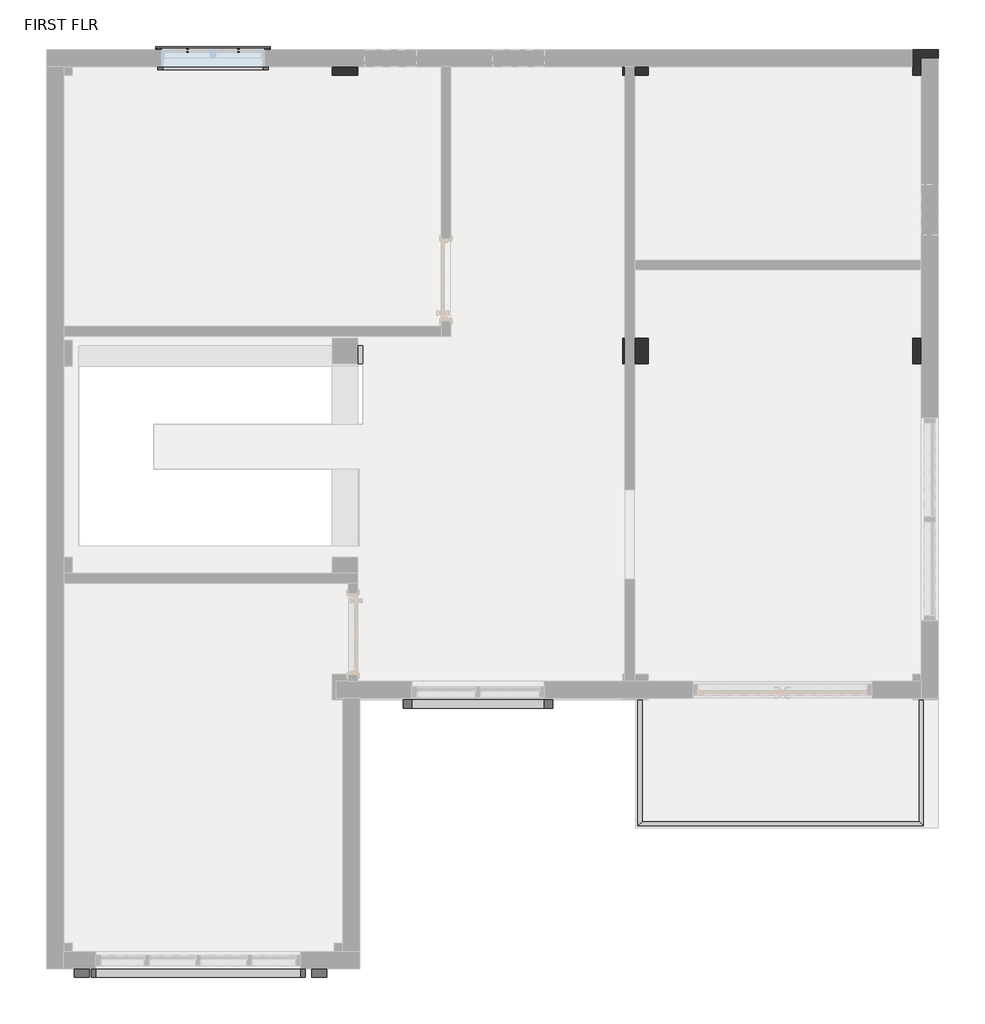
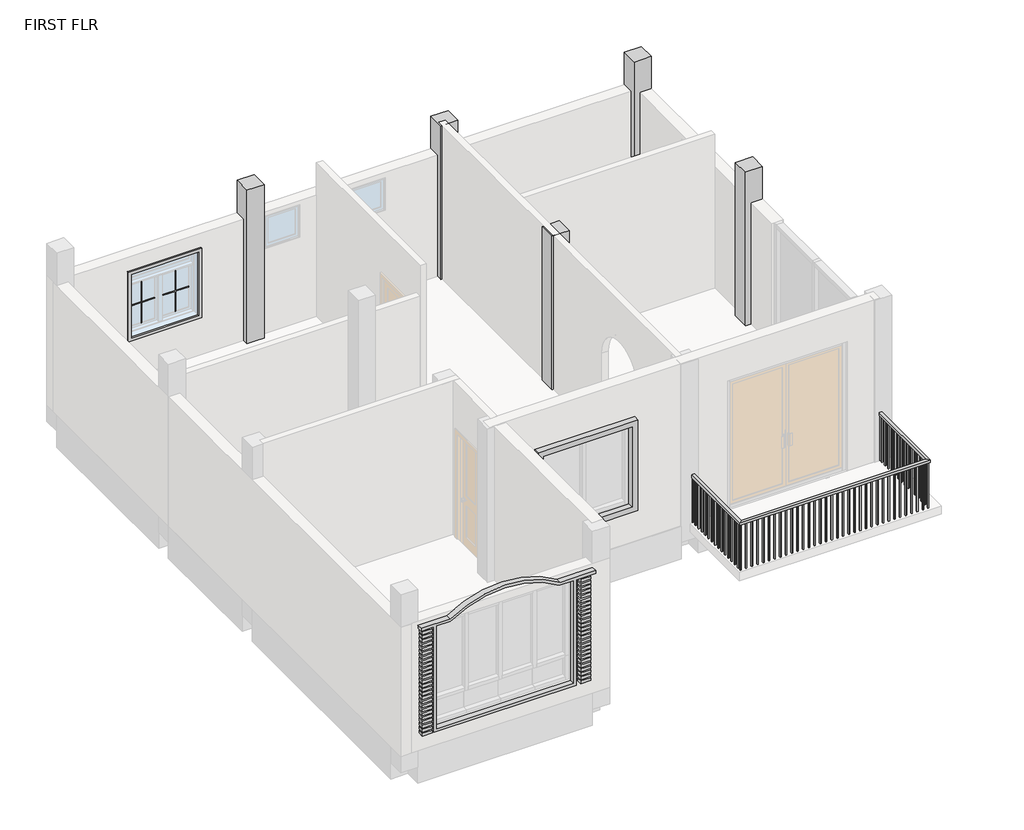
# One storey, part 3 of 3: 7 proxies, 6 beams, 5 columns, 1 railing.
"""IFC4 building model written with IfcOpenShell, lengths in millimetres."""

from ifc_helpers import new_model, si_unit, frame, origin, place, context, project, spatial, polyline, outline, extrude, faceted_brep, transform, mapped, element, save
from components import generic_models_5_generic_models_5_33064adf, generic_models_6_generic_models_6_eab10de4, generic_models_8_generic_models_8_74760410, muntin_pattern_2x2_muntin_pattern_2x2_2357e71d, muntin_pattern_2x2_muntin_pattern_2x2_302d8f29, trim_window_exterior_flat_with_sill_7cfdd449, trim_window_interior_flat_picture_frame_f1e0b15b

model = new_model("IFC4")

# Units and contexts
model_context = context("Model", 3, world=origin())
ifc_project = project(units=[si_unit("LENGTHUNIT", "METRE", prefix="MILLI")], contexts=[model_context])

# Site, building, storey
site = spatial("IfcSite", under=ifc_project)
building = spatial("IfcBuilding", under=site)
storey = spatial("IfcBuildingStorey", under=building, Name="FIRST FLR", Elevation=3352.8)

# Beams
placement = place(None, origin())
element("IfcBeam", 1, ObjectType="Concrete-Rectangular Beam : 12 x 24", at=placement, inside=storey, context=model_context, shape_type="Brep", body=[
    faceted_brep([(-4797.1270642, -2868.8747117, 3352.8), (-4797.1270642, -2564.0747117, 3352.8), (-7946.7270642, -2564.0747117, 3352.8), (-7946.7270642, -2868.8747117, 3352.8), (-4797.1270642, -2868.8747117, 2743.2), (-4797.1270642, -2868.8747117, 3048.0), (-7946.7270642, -2868.8747117, 3048.0), (-7946.7270642, -2868.8747117, 2743.2), (-4797.1270642, -2564.0747117, 2743.2), (-7946.7270642, -2564.0747117, 2743.2), (-4797.1270642, -2564.0747117, 3048.0), (-7946.7270642, -2564.0747117, 3048.0)], [[[0, 1, 2, 3]], [[4, 5, 0, 3, 6, 7]], [[8, 4, 7, 9]], [[1, 10, 8, 9, 11, 2]], [[2, 11, 9, 7, 6, 3]], [[1, 0, 5, 4, 8, 10]]]),
])
element("IfcBeam", 2, ObjectType="Concrete-Rectangular Beam : 12 x 24", at=placement, inside=storey, context=model_context, shape_type="Brep", body=[
    faceted_brep([(-1351.9658472, -2868.8747117, 3352.8), (-1351.9658472, -2564.0747117, 3352.8), (-4492.3270642, -2564.0747117, 3352.8), (-4492.3270642, -2868.8747117, 3352.8), (-1351.9658472, -2868.8747117, 2743.2), (-1351.9658472, -2868.8747117, 3048.0), (-4492.3270642, -2868.8747117, 3048.0), (-4492.3270642, -2868.8747117, 2743.2), (-1351.9658472, -2564.0747117, 2743.2), (-4492.3270642, -2564.0747117, 2743.2), (-1351.9658472, -2564.0747117, 3048.0), (-4492.3270642, -2564.0747117, 3048.0)], [[[0, 1, 2, 3]], [[4, 5, 0, 3, 6, 7]], [[8, 4, 7, 9]], [[1, 10, 8, 9, 11, 2]], [[2, 11, 9, 7, 6, 3]], [[1, 0, 5, 4, 8, 10]]]),
])
element("IfcBeam", 3, ObjectType="Concrete-Rectangular Beam : 12 x 24", at=placement, inside=storey, context=model_context, shape_type="Brep", body=[
    faceted_brep([(-1351.9658472, -5993.0747117, 3352.8), (-1047.1658472, -5993.0747117, 3352.8), (-1047.1658472, -2868.8747117, 3352.8), (-1351.9658472, -2868.8747117, 3352.8), (-1351.9658472, -5993.0747117, 2743.2), (-1351.9658472, -5993.0747117, 3048.0), (-1351.9658472, -2868.8747117, 3048.0), (-1351.9658472, -2868.8747117, 2743.2), (-1047.1658472, -5993.0747117, 2743.2), (-1047.1658472, -2868.8747117, 2743.2), (-1047.1658472, -5993.0747117, 3048.0), (-1047.1658472, -2868.8747117, 3048.0)], [[[0, 1, 2, 3]], [[4, 5, 0, 3, 6, 7]], [[8, 4, 7, 9]], [[1, 10, 8, 9, 11, 2]], [[2, 11, 9, 7, 6, 3]], [[1, 0, 5, 4, 8, 10]]]),
])
element("IfcBeam", 4, ObjectType="Concrete-Rectangular Beam : 12 x 24", at=placement, inside=storey, context=model_context, shape_type="Brep", body=[
    faceted_brep([(-4492.3270642, -5993.0747117, 3352.8), (-4492.3270642, -6297.8747117, 3352.8), (-1351.9658472, -6297.8747117, 3352.8), (-1351.9658472, -5993.0747117, 3352.8), (-4492.3270642, -5993.0747117, 2743.2), (-4492.3270642, -5993.0747117, 3048.0), (-1351.9658472, -5993.0747117, 3048.0), (-1351.9658472, -5993.0747117, 2743.2), (-4492.3270642, -6297.8747117, 2743.2), (-1351.9658472, -6297.8747117, 2743.2), (-4492.3270642, -6297.8747117, 3048.0), (-1351.9658472, -6297.8747117, 3048.0)], [[[0, 1, 2, 3]], [[4, 5, 0, 3, 6, 7]], [[8, 4, 7, 9]], [[1, 10, 8, 9, 11, 2]], [[2, 11, 9, 7, 6, 3]], [[1, 0, 5, 4, 8, 10]]]),
])
element("IfcBeam", 5, ObjectType="Concrete-Rectangular Beam : 12 x 24", at=placement, inside=storey, context=model_context, shape_type="Brep", body=[
    faceted_brep([(-4492.3270642, -2868.8747117, 3352.8), (-4797.1270642, -2868.8747117, 3352.8), (-4797.1270642, -5993.0747117, 3352.8), (-4492.3270642, -5993.0747117, 3352.8), (-4492.3270642, -2868.8747117, 2743.2), (-4492.3270642, -2868.8747117, 3048.0), (-4492.3270642, -5993.0747117, 3048.0), (-4492.3270642, -5993.0747117, 2743.2), (-4797.1270642, -2868.8747117, 2743.2), (-4797.1270642, -5993.0747117, 2743.2), (-4797.1270642, -2868.8747117, 3048.0), (-4797.1270642, -5993.0747117, 3048.0)], [[[0, 1, 2, 3]], [[4, 5, 0, 3, 6, 7]], [[8, 4, 7, 9]], [[1, 10, 8, 9, 11, 2]], [[1, 0, 5, 4, 8, 10]], [[2, 11, 9, 7, 6, 3]]]),
])
element("IfcBeam", 6, ObjectType="Concrete-Rectangular Beam : 12 x 24", at=placement, inside=storey, context=model_context, shape_type="Brep", body=[
    faceted_brep([(-4797.1270642, -6297.8747117, 3352.8), (-4797.1270642, -5993.0747117, 3352.8), (-7946.7270642, -5993.0747117, 3352.8), (-7946.7270642, -6297.8747117, 3352.8), (-7889.5770642, -6297.8747117, 3352.8), (-4801.7464557, -6297.8747117, 3352.8), (-4797.1270642, -6297.8747117, 2743.2), (-4797.1270642, -6297.8747117, 3048.0), (-7946.7270642, -6297.8747117, 3048.0), (-7946.7270642, -6297.8747117, 2743.2), (-4797.1270642, -5993.0747117, 2743.2), (-7946.7270642, -5993.0747117, 2743.2), (-4797.1270642, -5993.0747117, 3048.0), (-7946.7270642, -5993.0747117, 3048.0)], [[[0, 1, 2, 3, 4, 5]], [[6, 7, 0, 5, 4, 3, 8, 9]], [[10, 6, 9, 11]], [[1, 12, 10, 11, 13, 2]], [[1, 0, 7, 6, 10, 12]], [[3, 2, 13, 11, 9, 8]]]),
])

# Proxies
generic_models_5_generic_models_5_shape = generic_models_5_generic_models_5_33064adf(model_context)
element("IfcBuildingElementProxy", 7, Name="Generic Models 5 : Generic Models 5", ObjectType="Generic Models 5 : Generic Models 5", at=placement, inside=storey, context=model_context, shape_type="MappedRepresentation", body=[
    mapped(generic_models_5_generic_models_5_shape, transform((0.0, 0.0, 0.0), x_axis=(1.0, 0.0, 0.0), y_axis=(0.0, 1.0, 0.0), z_axis=(0.0, 0.0, 1.0))),
])
generic_models_6_generic_models_6_shape = generic_models_6_generic_models_6_eab10de4(model_context)
element("IfcBuildingElementProxy", 8, Name="Generic Models 6 : Generic Models 6", ObjectType="Generic Models 6 : Generic Models 6", at=placement, inside=storey, context=model_context, shape_type="MappedRepresentation", body=[
    mapped(generic_models_6_generic_models_6_shape, transform((0.0, 0.0, 0.0), x_axis=(1.0, 0.0, 0.0), y_axis=(0.0, 1.0, 0.0), z_axis=(0.0, 0.0, 1.0))),
])
generic_models_8_generic_models_8_shape = generic_models_8_generic_models_8_74760410(model_context)
element("IfcBuildingElementProxy", 9, Name="Generic Models 8 : Generic Models 8", ObjectType="Generic Models 8 : Generic Models 8", at=placement, inside=storey, context=model_context, shape_type="MappedRepresentation", body=[
    mapped(generic_models_8_generic_models_8_shape, transform((0.0, 0.0, 0.0), x_axis=(1.0, 0.0, 0.0), y_axis=(0.0, 1.0, 0.0), z_axis=(0.0, 0.0, 1.0))),
])
muntin_pattern_2x2_muntin_pattern_2x2_shape = muntin_pattern_2x2_muntin_pattern_2x2_2357e71d(model_context)
element("IfcBuildingElementProxy", 10, Name="Muntin Pattern_2x2 : Muntin Pattern_2x2", ObjectType="Muntin Pattern_2x2 : Muntin Pattern_2x2", at=placement, inside=storey, context=model_context, shape_type="MappedRepresentation", body=[
    mapped(muntin_pattern_2x2_muntin_pattern_2x2_shape, transform((-9970.7895642, -2573.5997117, 4337.05), x_axis=(1.0, 0.0, 0.0), y_axis=(0.0, 1.0, 0.0), z_axis=(0.0, 0.0, 1.0))),
])
muntin_pattern_2x2_muntin_pattern_2x2_2_shape = muntin_pattern_2x2_muntin_pattern_2x2_302d8f29(model_context)
element("IfcBuildingElementProxy", 11, Name="Muntin Pattern_2x2 : Muntin Pattern_2x2", ObjectType="Muntin Pattern_2x2 : Muntin Pattern_2x2", at=placement, inside=storey, context=model_context, shape_type="MappedRepresentation", body=[
    mapped(muntin_pattern_2x2_muntin_pattern_2x2_2_shape, transform((-9364.3645642, -2573.5997117, 4337.05), x_axis=(-1.0, 0.0, 0.0), y_axis=(0.0, -1.0, 0.0), z_axis=(0.0, 0.0, 1.0))),
])
trim_window_exterior_flat_with_sill_shape = trim_window_exterior_flat_with_sill_7cfdd449(model_context)
element("IfcBuildingElementProxy", 12, Name="Trim-Window-Exterior-Flat : with Sill", ObjectType="Trim-Window-Exterior-Flat : with Sill", at=placement, inside=storey, context=model_context, shape_type="MappedRepresentation", body=[
    mapped(trim_window_exterior_flat_with_sill_shape, transform((-9667.5770642, -2564.0747117, 5486.4), x_axis=(-1.0, 0.0, 0.0), y_axis=(0.0, 0.0, 1.0), z_axis=(0.0, 1.0, 0.0))),
])
trim_window_interior_flat_picture_frame_shape = trim_window_interior_flat_picture_frame_f1e0b15b(model_context)
element("IfcBuildingElementProxy", 13, Name="Trim-Window-Interior-Flat : Picture Frame", ObjectType="Trim-Window-Interior-Flat : Picture Frame", at=placement, inside=storey, context=model_context, shape_type="MappedRepresentation", body=[
    mapped(trim_window_interior_flat_picture_frame_shape, transform((-9667.5770642, -2767.2747117, 5486.4), x_axis=(1.0, 0.0, 0.0), y_axis=(0.0, 0.0, 1.0), z_axis=(0.0, -1.0, 0.0))),
])

# Columns
element("IfcColumn", 14, ObjectType="Concrete-Rectangular-Column : 12\" X 12\" COLUMN", at=placement, inside=storey, context=model_context, shape_type="Brep", body=[
    faceted_brep([(-7946.7270642, -2564.0747117, 3048.0), (-7946.7270642, -2868.8747117, 3048.0), (-8251.5270642, -2868.8747117, 3048.0), (-8251.5270642, -2564.0747117, 3048.0), (-7946.7270642, -2564.0747117, 6400.8), (-7946.7270642, -2868.8747117, 6400.8), (-7946.7270642, -2868.8747117, 3352.8), (-7946.7270642, -2564.0747117, 3352.8), (-8251.5270642, -2868.8747117, 6400.8), (-8251.5270642, -2868.8747117, 3352.8), (-8251.5270642, -2564.0747117, 6400.8), (-8251.5270642, -2564.0747117, 3352.8)], [[[0, 1, 2, 3]], [[4, 5, 6, 1, 0, 7]], [[5, 8, 9, 2, 1, 6]], [[8, 10, 11, 3, 2, 9]], [[10, 4, 7, 0, 3, 11]], [[4, 10, 8, 5]]]),
])
element("IfcColumn", 15, ObjectType="Concrete-Rectangular-Column : 12\" X 12\" COLUMN", at=placement, inside=storey, context=model_context, shape_type="Brep", body=[
    faceted_brep([(-4492.3270642, -2564.0747117, 3048.0), (-4492.3270642, -2868.8747117, 3048.0), (-4797.1270642, -2868.8747117, 3048.0), (-4797.1270642, -2564.0747117, 3048.0), (-4492.3270642, -2564.0747117, 6400.8), (-4492.3270642, -2868.8747117, 6400.8), (-4492.3270642, -2868.8747117, 3352.8), (-4492.3270642, -2564.0747117, 3352.8), (-4797.1270642, -2868.8747117, 6400.8), (-4797.1270642, -2868.8747117, 3352.8), (-4797.1270642, -2564.0747117, 6400.8), (-4797.1270642, -2564.0747117, 3352.8)], [[[0, 1, 2, 3]], [[4, 5, 6, 1, 0, 7]], [[5, 8, 9, 2, 1, 6]], [[8, 10, 11, 3, 2, 9]], [[10, 4, 7, 0, 3, 11]], [[4, 10, 8, 5]]]),
])
element("IfcColumn", 16, ObjectType="Concrete-Rectangular-Column : 12\" X 12\" COLUMN", at=placement, inside=storey, context=model_context, shape_type="Brep", body=[
    faceted_brep([(-1047.1658472, -2564.0747117, 3048.0), (-1047.1658472, -2868.8747117, 3048.0), (-1351.9658472, -2868.8747117, 3048.0), (-1351.9658472, -2564.0747117, 3048.0), (-1047.1658472, -2564.0747117, 6400.8), (-1047.1658472, -2868.8747117, 6400.8), (-1047.1658472, -2868.8747117, 3352.8), (-1351.9658472, -2868.8747117, 6400.8), (-1351.9658472, -2868.8747117, 3352.8), (-1351.9658472, -2564.0747117, 6400.8), (-1351.9658472, -2564.0747117, 3352.8)], [[[0, 1, 2, 3]], [[4, 5, 6, 1, 0]], [[5, 7, 8, 2, 1, 6]], [[7, 9, 10, 3, 2, 8]], [[9, 4, 0, 3, 10]], [[4, 9, 7, 5]]]),
])
element("IfcColumn", 17, ObjectType="Concrete-Rectangular-Column : 12\" X 12\" COLUMN", at=placement, inside=storey, context=model_context, shape_type="Brep", body=[
    faceted_brep([(-1047.1658472, -5993.0747117, 3048.0), (-1047.1658472, -6297.8747117, 3048.0), (-1351.9658472, -6297.8747117, 3048.0), (-1351.9658472, -5993.0747117, 3048.0), (-1047.1658472, -5993.0747117, 6400.8), (-1047.1658472, -6297.8747117, 6400.8), (-1047.1658472, -6297.8747117, 3352.8), (-1047.1658472, -5993.0747117, 3352.8), (-1351.9658472, -6297.8747117, 6400.8), (-1351.9658472, -6297.8747117, 3352.8), (-1351.9658472, -5993.0747117, 6400.8), (-1351.9658472, -5993.0747117, 3352.8)], [[[0, 1, 2, 3]], [[4, 5, 6, 1, 0, 7]], [[5, 8, 9, 2, 1, 6]], [[8, 10, 11, 3, 2, 9]], [[10, 4, 7, 0, 3, 11]], [[4, 10, 8, 5]]]),
])
element("IfcColumn", 18, ObjectType="Concrete-Rectangular-Column : 12\" X 12\" COLUMN", at=placement, inside=storey, context=model_context, shape_type="Brep", body=[
    faceted_brep([(-4492.3270642, -5993.0747117, 3048.0), (-4492.3270642, -6297.8747117, 3048.0), (-4797.1270642, -6297.8747117, 3048.0), (-4797.1270642, -5993.0747117, 3048.0), (-4492.3270642, -5993.0747117, 6400.8), (-4492.3270642, -6297.8747117, 6400.8), (-4492.3270642, -6297.8747117, 3352.8), (-4492.3270642, -5993.0747117, 3352.8), (-4797.1270642, -6297.8747117, 6400.8), (-4797.1270642, -6297.8747117, 3352.8), (-4797.1270642, -5993.0747117, 6400.8), (-4797.1270642, -5993.0747117, 3352.8)], [[[0, 1, 2, 3]], [[4, 5, 6, 1, 0, 7]], [[5, 8, 9, 2, 1, 6]], [[8, 10, 11, 3, 2, 9]], [[10, 4, 7, 0, 3, 11]], [[4, 10, 8, 5]]]),
])

# Railing
element("IfcRailing", 19, ObjectType="RAILINGS 6\"", at=placement, inside=storey, context=model_context, shape_type="SolidModel", body=[
    faceted_brep([(-4568.5270642, -10271.3896616, 4267.2), (-4568.5270642, -10271.3896616, 4216.4), (-4619.3270642, -10271.3896616, 4216.4), (-4619.3270642, -10271.3896616, 4267.2), (-4568.5270642, -11736.14549, 4267.2), (-4568.5270642, -11736.14549, 4216.4), (-4619.3270642, -11786.94549, 4216.4), (-4619.3270642, -11786.94549, 4267.2), (-1275.7658472, -11736.14549, 4267.2), (-1275.7658472, -11736.14549, 4216.4), (-1224.9658472, -11786.94549, 4216.4), (-1224.9658472, -11786.94549, 4267.2), (-1275.7658472, -10271.3896616, 4267.2), (-1224.9658472, -10271.3896616, 4267.2), (-1224.9658472, -10271.3896616, 4216.4), (-1275.7658472, -10271.3896616, 4216.4)], [[[0, 1, 2, 3]], [[1, 0, 4, 5]], [[2, 1, 5, 6]], [[3, 2, 6, 7]], [[0, 3, 7, 4]], [[5, 4, 8, 9]], [[6, 5, 9, 10]], [[7, 6, 10, 11]], [[4, 7, 11, 8]], [[12, 13, 14, 15]], [[9, 8, 12, 15]], [[10, 9, 15, 14]], [[11, 10, 14, 13]], [[8, 11, 13, 12]]]),
    extrude(outline(polyline([(-1240.8408472, -10348.67049), (-1259.8908472, -10348.67049), (-1259.8908472, -10329.62049), (-1240.8408472, -10329.62049), (-1240.8408472, -10348.67049)])), frame((0.0, 0.0, 3352.8), z_axis=(0.0, 0.0, 1.0), x_axis=(1.0, 0.0, 0.0)), (0.0, 0.0, 1.0), 863.6),
    extrude(outline(polyline([(-1240.8408472, -10450.27049), (-1259.8908472, -10450.27049), (-1259.8908472, -10431.22049), (-1240.8408472, -10431.22049), (-1240.8408472, -10450.27049)])), frame((0.0, 0.0, 3352.8), z_axis=(0.0, 0.0, 1.0), x_axis=(1.0, 0.0, 0.0)), (0.0, 0.0, 1.0), 863.6),
    extrude(outline(polyline([(-1240.8408472, -10551.87049), (-1259.8908472, -10551.87049), (-1259.8908472, -10532.82049), (-1240.8408472, -10532.82049), (-1240.8408472, -10551.87049)])), frame((0.0, 0.0, 3352.8), z_axis=(0.0, 0.0, 1.0), x_axis=(1.0, 0.0, 0.0)), (0.0, 0.0, 1.0), 863.6),
    extrude(outline(polyline([(-1240.8408472, -10653.47049), (-1259.8908472, -10653.47049), (-1259.8908472, -10634.42049), (-1240.8408472, -10634.42049), (-1240.8408472, -10653.47049)])), frame((0.0, 0.0, 3352.8), z_axis=(0.0, 0.0, 1.0), x_axis=(1.0, 0.0, 0.0)), (0.0, 0.0, 1.0), 863.6),
    extrude(outline(polyline([(-1240.8408472, -10755.07049), (-1259.8908472, -10755.07049), (-1259.8908472, -10736.02049), (-1240.8408472, -10736.02049), (-1240.8408472, -10755.07049)])), frame((0.0, 0.0, 3352.8), z_axis=(0.0, 0.0, 1.0), x_axis=(1.0, 0.0, 0.0)), (0.0, 0.0, 1.0), 863.6),
    extrude(outline(polyline([(-1240.8408472, -10856.67049), (-1259.8908472, -10856.67049), (-1259.8908472, -10837.62049), (-1240.8408472, -10837.62049), (-1240.8408472, -10856.67049)])), frame((0.0, 0.0, 3352.8), z_axis=(0.0, 0.0, 1.0), x_axis=(1.0, 0.0, 0.0)), (0.0, 0.0, 1.0), 863.6),
    extrude(outline(polyline([(-1240.8408472, -10958.27049), (-1259.8908472, -10958.27049), (-1259.8908472, -10939.22049), (-1240.8408472, -10939.22049), (-1240.8408472, -10958.27049)])), frame((0.0, 0.0, 3352.8), z_axis=(0.0, 0.0, 1.0), x_axis=(1.0, 0.0, 0.0)), (0.0, 0.0, 1.0), 863.6),
    extrude(outline(polyline([(-1240.8408472, -11059.87049), (-1259.8908472, -11059.87049), (-1259.8908472, -11040.82049), (-1240.8408472, -11040.82049), (-1240.8408472, -11059.87049)])), frame((0.0, 0.0, 3352.8), z_axis=(0.0, 0.0, 1.0), x_axis=(1.0, 0.0, 0.0)), (0.0, 0.0, 1.0), 863.6),
    extrude(outline(polyline([(-1240.8408472, -11161.47049), (-1259.8908472, -11161.47049), (-1259.8908472, -11142.42049), (-1240.8408472, -11142.42049), (-1240.8408472, -11161.47049)])), frame((0.0, 0.0, 3352.8), z_axis=(0.0, 0.0, 1.0), x_axis=(1.0, 0.0, 0.0)), (0.0, 0.0, 1.0), 863.6),
    extrude(outline(polyline([(-1240.8408472, -11263.07049), (-1259.8908472, -11263.07049), (-1259.8908472, -11244.02049), (-1240.8408472, -11244.02049), (-1240.8408472, -11263.07049)])), frame((0.0, 0.0, 3352.8), z_axis=(0.0, 0.0, 1.0), x_axis=(1.0, 0.0, 0.0)), (0.0, 0.0, 1.0), 863.6),
    extrude(outline(polyline([(-1240.8408472, -11364.67049), (-1259.8908472, -11364.67049), (-1259.8908472, -11345.62049), (-1240.8408472, -11345.62049), (-1240.8408472, -11364.67049)])), frame((0.0, 0.0, 3352.8), z_axis=(0.0, 0.0, 1.0), x_axis=(1.0, 0.0, 0.0)), (0.0, 0.0, 1.0), 863.6),
    extrude(outline(polyline([(-1240.8408472, -11466.27049), (-1259.8908472, -11466.27049), (-1259.8908472, -11447.22049), (-1240.8408472, -11447.22049), (-1240.8408472, -11466.27049)])), frame((0.0, 0.0, 3352.8), z_axis=(0.0, 0.0, 1.0), x_axis=(1.0, 0.0, 0.0)), (0.0, 0.0, 1.0), 863.6),
    extrude(outline(polyline([(-1240.8408472, -11567.87049), (-1259.8908472, -11567.87049), (-1259.8908472, -11548.82049), (-1240.8408472, -11548.82049), (-1240.8408472, -11567.87049)])), frame((0.0, 0.0, 3352.8), z_axis=(0.0, 0.0, 1.0), x_axis=(1.0, 0.0, 0.0)), (0.0, 0.0, 1.0), 863.6),
    extrude(outline(polyline([(-1240.8408472, -11669.47049), (-1259.8908472, -11669.47049), (-1259.8908472, -11650.42049), (-1240.8408472, -11650.42049), (-1240.8408472, -11669.47049)])), frame((0.0, 0.0, 3352.8), z_axis=(0.0, 0.0, 1.0), x_axis=(1.0, 0.0, 0.0)), (0.0, 0.0, 1.0), 863.6),
    extrude(outline(polyline([(-1352.2520642, -11771.07049), (-1352.2520642, -11752.02049), (-1333.2020642, -11752.02049), (-1333.2020642, -11771.07049), (-1352.2520642, -11771.07049)])), frame((0.0, 0.0, 3352.8), z_axis=(0.0, 0.0, 1.0), x_axis=(1.0, 0.0, 0.0)), (0.0, 0.0, 1.0), 863.6),
    extrude(outline(polyline([(-1453.8520642, -11771.07049), (-1453.8520642, -11752.02049), (-1434.8020642, -11752.02049), (-1434.8020642, -11771.07049), (-1453.8520642, -11771.07049)])), frame((0.0, 0.0, 3352.8), z_axis=(0.0, 0.0, 1.0), x_axis=(1.0, 0.0, 0.0)), (0.0, 0.0, 1.0), 863.6),
    extrude(outline(polyline([(-1555.4520642, -11771.07049), (-1555.4520642, -11752.02049), (-1536.4020642, -11752.02049), (-1536.4020642, -11771.07049), (-1555.4520642, -11771.07049)])), frame((0.0, 0.0, 3352.8), z_axis=(0.0, 0.0, 1.0), x_axis=(1.0, 0.0, 0.0)), (0.0, 0.0, 1.0), 863.6),
    extrude(outline(polyline([(-1657.0520642, -11771.07049), (-1657.0520642, -11752.02049), (-1638.0020642, -11752.02049), (-1638.0020642, -11771.07049), (-1657.0520642, -11771.07049)])), frame((0.0, 0.0, 3352.8), z_axis=(0.0, 0.0, 1.0), x_axis=(1.0, 0.0, 0.0)), (0.0, 0.0, 1.0), 863.6),
    extrude(outline(polyline([(-1758.6520642, -11771.07049), (-1758.6520642, -11752.02049), (-1739.6020642, -11752.02049), (-1739.6020642, -11771.07049), (-1758.6520642, -11771.07049)])), frame((0.0, 0.0, 3352.8), z_axis=(0.0, 0.0, 1.0), x_axis=(1.0, 0.0, 0.0)), (0.0, 0.0, 1.0), 863.6),
    extrude(outline(polyline([(-1860.2520642, -11771.07049), (-1860.2520642, -11752.02049), (-1841.2020642, -11752.02049), (-1841.2020642, -11771.07049), (-1860.2520642, -11771.07049)])), frame((0.0, 0.0, 3352.8), z_axis=(0.0, 0.0, 1.0), x_axis=(1.0, 0.0, 0.0)), (0.0, 0.0, 1.0), 863.6),
    extrude(outline(polyline([(-1961.8520642, -11771.07049), (-1961.8520642, -11752.02049), (-1942.8020642, -11752.02049), (-1942.8020642, -11771.07049), (-1961.8520642, -11771.07049)])), frame((0.0, 0.0, 3352.8), z_axis=(0.0, 0.0, 1.0), x_axis=(1.0, 0.0, 0.0)), (0.0, 0.0, 1.0), 863.6),
    extrude(outline(polyline([(-2063.4520642, -11771.07049), (-2063.4520642, -11752.02049), (-2044.4020642, -11752.02049), (-2044.4020642, -11771.07049), (-2063.4520642, -11771.07049)])), frame((0.0, 0.0, 3352.8), z_axis=(0.0, 0.0, 1.0), x_axis=(1.0, 0.0, 0.0)), (0.0, 0.0, 1.0), 863.6),
    extrude(outline(polyline([(-2165.0520642, -11771.07049), (-2165.0520642, -11752.02049), (-2146.0020642, -11752.02049), (-2146.0020642, -11771.07049), (-2165.0520642, -11771.07049)])), frame((0.0, 0.0, 3352.8), z_axis=(0.0, 0.0, 1.0), x_axis=(1.0, 0.0, 0.0)), (0.0, 0.0, 1.0), 863.6),
    extrude(outline(polyline([(-2266.6520642, -11771.07049), (-2266.6520642, -11752.02049), (-2247.6020642, -11752.02049), (-2247.6020642, -11771.07049), (-2266.6520642, -11771.07049)])), frame((0.0, 0.0, 3352.8), z_axis=(0.0, 0.0, 1.0), x_axis=(1.0, 0.0, 0.0)), (0.0, 0.0, 1.0), 863.6),
    extrude(outline(polyline([(-2368.2520642, -11771.07049), (-2368.2520642, -11752.02049), (-2349.2020642, -11752.02049), (-2349.2020642, -11771.07049), (-2368.2520642, -11771.07049)])), frame((0.0, 0.0, 3352.8), z_axis=(0.0, 0.0, 1.0), x_axis=(1.0, 0.0, 0.0)), (0.0, 0.0, 1.0), 863.6),
    extrude(outline(polyline([(-2469.8520642, -11771.07049), (-2469.8520642, -11752.02049), (-2450.8020642, -11752.02049), (-2450.8020642, -11771.07049), (-2469.8520642, -11771.07049)])), frame((0.0, 0.0, 3352.8), z_axis=(0.0, 0.0, 1.0), x_axis=(1.0, 0.0, 0.0)), (0.0, 0.0, 1.0), 863.6),
    extrude(outline(polyline([(-2571.4520642, -11771.07049), (-2571.4520642, -11752.02049), (-2552.4020642, -11752.02049), (-2552.4020642, -11771.07049), (-2571.4520642, -11771.07049)])), frame((0.0, 0.0, 3352.8), z_axis=(0.0, 0.0, 1.0), x_axis=(1.0, 0.0, 0.0)), (0.0, 0.0, 1.0), 863.6),
    extrude(outline(polyline([(-2673.0520642, -11771.07049), (-2673.0520642, -11752.02049), (-2654.0020642, -11752.02049), (-2654.0020642, -11771.07049), (-2673.0520642, -11771.07049)])), frame((0.0, 0.0, 3352.8), z_axis=(0.0, 0.0, 1.0), x_axis=(1.0, 0.0, 0.0)), (0.0, 0.0, 1.0), 863.6),
    extrude(outline(polyline([(-2774.6520642, -11771.07049), (-2774.6520642, -11752.02049), (-2755.6020642, -11752.02049), (-2755.6020642, -11771.07049), (-2774.6520642, -11771.07049)])), frame((0.0, 0.0, 3352.8), z_axis=(0.0, 0.0, 1.0), x_axis=(1.0, 0.0, 0.0)), (0.0, 0.0, 1.0), 863.6),
    extrude(outline(polyline([(-2876.2520642, -11771.07049), (-2876.2520642, -11752.02049), (-2857.2020642, -11752.02049), (-2857.2020642, -11771.07049), (-2876.2520642, -11771.07049)])), frame((0.0, 0.0, 3352.8), z_axis=(0.0, 0.0, 1.0), x_axis=(1.0, 0.0, 0.0)), (0.0, 0.0, 1.0), 863.6),
    extrude(outline(polyline([(-2977.8520642, -11771.07049), (-2977.8520642, -11752.02049), (-2958.8020642, -11752.02049), (-2958.8020642, -11771.07049), (-2977.8520642, -11771.07049)])), frame((0.0, 0.0, 3352.8), z_axis=(0.0, 0.0, 1.0), x_axis=(1.0, 0.0, 0.0)), (0.0, 0.0, 1.0), 863.6),
    extrude(outline(polyline([(-3079.4520642, -11771.07049), (-3079.4520642, -11752.02049), (-3060.4020642, -11752.02049), (-3060.4020642, -11771.07049), (-3079.4520642, -11771.07049)])), frame((0.0, 0.0, 3352.8), z_axis=(0.0, 0.0, 1.0), x_axis=(1.0, 0.0, 0.0)), (0.0, 0.0, 1.0), 863.6),
    extrude(outline(polyline([(-3181.0520642, -11771.07049), (-3181.0520642, -11752.02049), (-3162.0020642, -11752.02049), (-3162.0020642, -11771.07049), (-3181.0520642, -11771.07049)])), frame((0.0, 0.0, 3352.8), z_axis=(0.0, 0.0, 1.0), x_axis=(1.0, 0.0, 0.0)), (0.0, 0.0, 1.0), 863.6),
    extrude(outline(polyline([(-3282.6520642, -11771.07049), (-3282.6520642, -11752.02049), (-3263.6020642, -11752.02049), (-3263.6020642, -11771.07049), (-3282.6520642, -11771.07049)])), frame((0.0, 0.0, 3352.8), z_axis=(0.0, 0.0, 1.0), x_axis=(1.0, 0.0, 0.0)), (0.0, 0.0, 1.0), 863.6),
    extrude(outline(polyline([(-3384.2520642, -11771.07049), (-3384.2520642, -11752.02049), (-3365.2020642, -11752.02049), (-3365.2020642, -11771.07049), (-3384.2520642, -11771.07049)])), frame((0.0, 0.0, 3352.8), z_axis=(0.0, 0.0, 1.0), x_axis=(1.0, 0.0, 0.0)), (0.0, 0.0, 1.0), 863.6),
    extrude(outline(polyline([(-3485.8520642, -11771.07049), (-3485.8520642, -11752.02049), (-3466.8020642, -11752.02049), (-3466.8020642, -11771.07049), (-3485.8520642, -11771.07049)])), frame((0.0, 0.0, 3352.8), z_axis=(0.0, 0.0, 1.0), x_axis=(1.0, 0.0, 0.0)), (0.0, 0.0, 1.0), 863.6),
    extrude(outline(polyline([(-3587.4520642, -11771.07049), (-3587.4520642, -11752.02049), (-3568.4020642, -11752.02049), (-3568.4020642, -11771.07049), (-3587.4520642, -11771.07049)])), frame((0.0, 0.0, 3352.8), z_axis=(0.0, 0.0, 1.0), x_axis=(1.0, 0.0, 0.0)), (0.0, 0.0, 1.0), 863.6),
    extrude(outline(polyline([(-3689.0520642, -11771.07049), (-3689.0520642, -11752.02049), (-3670.0020642, -11752.02049), (-3670.0020642, -11771.07049), (-3689.0520642, -11771.07049)])), frame((0.0, 0.0, 3352.8), z_axis=(0.0, 0.0, 1.0), x_axis=(1.0, 0.0, 0.0)), (0.0, 0.0, 1.0), 863.6),
    extrude(outline(polyline([(-3790.6520642, -11771.07049), (-3790.6520642, -11752.02049), (-3771.6020642, -11752.02049), (-3771.6020642, -11771.07049), (-3790.6520642, -11771.07049)])), frame((0.0, 0.0, 3352.8), z_axis=(0.0, 0.0, 1.0), x_axis=(1.0, 0.0, 0.0)), (0.0, 0.0, 1.0), 863.6),
    extrude(outline(polyline([(-3892.2520642, -11771.07049), (-3892.2520642, -11752.02049), (-3873.2020642, -11752.02049), (-3873.2020642, -11771.07049), (-3892.2520642, -11771.07049)])), frame((0.0, 0.0, 3352.8), z_axis=(0.0, 0.0, 1.0), x_axis=(1.0, 0.0, 0.0)), (0.0, 0.0, 1.0), 863.6),
    extrude(outline(polyline([(-3993.8520642, -11771.07049), (-3993.8520642, -11752.02049), (-3974.8020642, -11752.02049), (-3974.8020642, -11771.07049), (-3993.8520642, -11771.07049)])), frame((0.0, 0.0, 3352.8), z_axis=(0.0, 0.0, 1.0), x_axis=(1.0, 0.0, 0.0)), (0.0, 0.0, 1.0), 863.6),
    extrude(outline(polyline([(-4095.4520642, -11771.07049), (-4095.4520642, -11752.02049), (-4076.4020642, -11752.02049), (-4076.4020642, -11771.07049), (-4095.4520642, -11771.07049)])), frame((0.0, 0.0, 3352.8), z_axis=(0.0, 0.0, 1.0), x_axis=(1.0, 0.0, 0.0)), (0.0, 0.0, 1.0), 863.6),
    extrude(outline(polyline([(-4197.0520642, -11771.07049), (-4197.0520642, -11752.02049), (-4178.0020642, -11752.02049), (-4178.0020642, -11771.07049), (-4197.0520642, -11771.07049)])), frame((0.0, 0.0, 3352.8), z_axis=(0.0, 0.0, 1.0), x_axis=(1.0, 0.0, 0.0)), (0.0, 0.0, 1.0), 863.6),
    extrude(outline(polyline([(-4298.6520642, -11771.07049), (-4298.6520642, -11752.02049), (-4279.6020642, -11752.02049), (-4279.6020642, -11771.07049), (-4298.6520642, -11771.07049)])), frame((0.0, 0.0, 3352.8), z_axis=(0.0, 0.0, 1.0), x_axis=(1.0, 0.0, 0.0)), (0.0, 0.0, 1.0), 863.6),
    extrude(outline(polyline([(-4400.2520642, -11771.07049), (-4400.2520642, -11752.02049), (-4381.2020642, -11752.02049), (-4381.2020642, -11771.07049), (-4400.2520642, -11771.07049)])), frame((0.0, 0.0, 3352.8), z_axis=(0.0, 0.0, 1.0), x_axis=(1.0, 0.0, 0.0)), (0.0, 0.0, 1.0), 863.6),
    extrude(outline(polyline([(-4501.8520642, -11771.07049), (-4501.8520642, -11752.02049), (-4482.8020642, -11752.02049), (-4482.8020642, -11771.07049), (-4501.8520642, -11771.07049)])), frame((0.0, 0.0, 3352.8), z_axis=(0.0, 0.0, 1.0), x_axis=(1.0, 0.0, 0.0)), (0.0, 0.0, 1.0), 863.6),
    extrude(outline(polyline([(-4603.4520642, -11684.2646616), (-4584.4020642, -11684.2646616), (-4584.4020642, -11703.3146616), (-4603.4520642, -11703.3146616), (-4603.4520642, -11684.2646616)])), frame((0.0, 0.0, 3352.8), z_axis=(0.0, 0.0, 1.0), x_axis=(1.0, 0.0, 0.0)), (0.0, 0.0, 1.0), 863.6),
    extrude(outline(polyline([(-4603.4520642, -11582.6646616), (-4584.4020642, -11582.6646616), (-4584.4020642, -11601.7146616), (-4603.4520642, -11601.7146616), (-4603.4520642, -11582.6646616)])), frame((0.0, 0.0, 3352.8), z_axis=(0.0, 0.0, 1.0), x_axis=(1.0, 0.0, 0.0)), (0.0, 0.0, 1.0), 863.6),
    extrude(outline(polyline([(-4603.4520642, -11481.0646616), (-4584.4020642, -11481.0646616), (-4584.4020642, -11500.1146616), (-4603.4520642, -11500.1146616), (-4603.4520642, -11481.0646616)])), frame((0.0, 0.0, 3352.8), z_axis=(0.0, 0.0, 1.0), x_axis=(1.0, 0.0, 0.0)), (0.0, 0.0, 1.0), 863.6),
    extrude(outline(polyline([(-4603.4520642, -11379.4646616), (-4584.4020642, -11379.4646616), (-4584.4020642, -11398.5146616), (-4603.4520642, -11398.5146616), (-4603.4520642, -11379.4646616)])), frame((0.0, 0.0, 3352.8), z_axis=(0.0, 0.0, 1.0), x_axis=(1.0, 0.0, 0.0)), (0.0, 0.0, 1.0), 863.6),
    extrude(outline(polyline([(-4603.4520642, -11277.8646616), (-4584.4020642, -11277.8646616), (-4584.4020642, -11296.9146616), (-4603.4520642, -11296.9146616), (-4603.4520642, -11277.8646616)])), frame((0.0, 0.0, 3352.8), z_axis=(0.0, 0.0, 1.0), x_axis=(1.0, 0.0, 0.0)), (0.0, 0.0, 1.0), 863.6),
    extrude(outline(polyline([(-4603.4520642, -11176.2646616), (-4584.4020642, -11176.2646616), (-4584.4020642, -11195.3146616), (-4603.4520642, -11195.3146616), (-4603.4520642, -11176.2646616)])), frame((0.0, 0.0, 3352.8), z_axis=(0.0, 0.0, 1.0), x_axis=(1.0, 0.0, 0.0)), (0.0, 0.0, 1.0), 863.6),
    extrude(outline(polyline([(-4603.4520642, -11074.6646616), (-4584.4020642, -11074.6646616), (-4584.4020642, -11093.7146616), (-4603.4520642, -11093.7146616), (-4603.4520642, -11074.6646616)])), frame((0.0, 0.0, 3352.8), z_axis=(0.0, 0.0, 1.0), x_axis=(1.0, 0.0, 0.0)), (0.0, 0.0, 1.0), 863.6),
    extrude(outline(polyline([(-4603.4520642, -10973.0646616), (-4584.4020642, -10973.0646616), (-4584.4020642, -10992.1146616), (-4603.4520642, -10992.1146616), (-4603.4520642, -10973.0646616)])), frame((0.0, 0.0, 3352.8), z_axis=(0.0, 0.0, 1.0), x_axis=(1.0, 0.0, 0.0)), (0.0, 0.0, 1.0), 863.6),
    extrude(outline(polyline([(-4603.4520642, -10871.4646616), (-4584.4020642, -10871.4646616), (-4584.4020642, -10890.5146616), (-4603.4520642, -10890.5146616), (-4603.4520642, -10871.4646616)])), frame((0.0, 0.0, 3352.8), z_axis=(0.0, 0.0, 1.0), x_axis=(1.0, 0.0, 0.0)), (0.0, 0.0, 1.0), 863.6),
    extrude(outline(polyline([(-4603.4520642, -10769.8646616), (-4584.4020642, -10769.8646616), (-4584.4020642, -10788.9146616), (-4603.4520642, -10788.9146616), (-4603.4520642, -10769.8646616)])), frame((0.0, 0.0, 3352.8), z_axis=(0.0, 0.0, 1.0), x_axis=(1.0, 0.0, 0.0)), (0.0, 0.0, 1.0), 863.6),
    extrude(outline(polyline([(-4603.4520642, -10668.2646616), (-4584.4020642, -10668.2646616), (-4584.4020642, -10687.3146616), (-4603.4520642, -10687.3146616), (-4603.4520642, -10668.2646616)])), frame((0.0, 0.0, 3352.8), z_axis=(0.0, 0.0, 1.0), x_axis=(1.0, 0.0, 0.0)), (0.0, 0.0, 1.0), 863.6),
    extrude(outline(polyline([(-4603.4520642, -10566.6646616), (-4584.4020642, -10566.6646616), (-4584.4020642, -10585.7146616), (-4603.4520642, -10585.7146616), (-4603.4520642, -10566.6646616)])), frame((0.0, 0.0, 3352.8), z_axis=(0.0, 0.0, 1.0), x_axis=(1.0, 0.0, 0.0)), (0.0, 0.0, 1.0), 863.6),
    extrude(outline(polyline([(-4603.4520642, -10465.0646616), (-4584.4020642, -10465.0646616), (-4584.4020642, -10484.1146616), (-4603.4520642, -10484.1146616), (-4603.4520642, -10465.0646616)])), frame((0.0, 0.0, 3352.8), z_axis=(0.0, 0.0, 1.0), x_axis=(1.0, 0.0, 0.0)), (0.0, 0.0, 1.0), 863.6),
    extrude(outline(polyline([(-4603.4520642, -10363.4646616), (-4584.4020642, -10363.4646616), (-4584.4020642, -10382.5146616), (-4603.4520642, -10382.5146616), (-4603.4520642, -10363.4646616)])), frame((0.0, 0.0, 3352.8), z_axis=(0.0, 0.0, 1.0), x_axis=(1.0, 0.0, 0.0)), (0.0, 0.0, 1.0), 863.6),
    extrude(outline(polyline([(-1259.8908472, -11771.07049), (-1259.8908472, -11752.02049), (-1240.8408472, -11752.02049), (-1240.8408472, -11771.07049), (-1259.8908472, -11771.07049)])), frame((0.0, 0.0, 3352.8), z_axis=(0.0, 0.0, 1.0), x_axis=(1.0, 0.0, 0.0)), (0.0, 0.0, 1.0), 863.6),
    extrude(outline(polyline([(-4603.4520642, -11752.02049), (-4584.4020642, -11752.02049), (-4584.4020642, -11771.07049), (-4603.4520642, -11771.07049), (-4603.4520642, -11752.02049)])), frame((0.0, 0.0, 3352.8), z_axis=(0.0, 0.0, 1.0), x_axis=(1.0, 0.0, 0.0)), (0.0, 0.0, 1.0), 863.6),
    extrude(outline(polyline([(-1240.8408472, -10290.4396616), (-1259.8908472, -10290.4396616), (-1259.8908472, -10271.3896616), (-1240.8408472, -10271.3896616), (-1240.8408472, -10290.4396616)])), frame((0.0, 0.0, 3352.8), z_axis=(0.0, 0.0, 1.0), x_axis=(1.0, 0.0, 0.0)), (0.0, 0.0, 1.0), 863.6),
    extrude(outline(polyline([(-4603.4520642, -10271.3896616), (-4584.4020642, -10271.3896616), (-4584.4020642, -10290.4396616), (-4603.4520642, -10290.4396616), (-4603.4520642, -10271.3896616)])), frame((0.0, 0.0, 3352.8), z_axis=(0.0, 0.0, 1.0), x_axis=(1.0, 0.0, 0.0)), (0.0, 0.0, 1.0), 863.6),
])

save(model, "model.ifc")

# Revit data of these elements
# Type "Concrete-Rectangular Beam : 12 x 24"
#   Assembly Code = "B10"
#   Length [instance default] = 5' - 0"
#   b = 1' - 0"
#   h = 2' - 0"
#   Structural Material [instance default] = Concrete, Cast-in-Place gray
# Type "Muntin Pattern_2x2 : Muntin Pattern_2x2"
#   Width [instance default] = 4' - 0"
#   Thickness = 0' - 0 1/2"
#   Height [instance default] = 4' - 0"
#   Distance = 0' - 0 3/4"
#   Interior Material [instance default] = none
#   Exterior Material [instance default] = none
#   Default Elevation = 0
# Type "Trim-Window-Exterior-Flat : with Sill"
#   Trim Width = 0' - 2 1/4"
#   Trim Thickness_Picture Frame = 0' - 1 1/4"
#   Trim Thickness_with Sill = 0' - 0 3/4"
#   Sill Thickness = 0' - 1 1/4"
#   Opening Width [instance default] = 2' - 0"
#   Opening Height [instance default] = 3' - 0"
#   Default Elevation = 4' - 0"
#   Sill = yes
#   Picture Frame = no
#   Trim Material [instance default] = none
# Type "Trim-Window-Interior-Flat : Picture Frame"
#   Trim Thickness_Picture Frame = 0' - 1 1/4"
#   Trim Width = 0' - 2 1/4"
#   Trim Thickness_with Sill = 0' - 0 3/4"
#   Sill Thickness = 0' - 1 1/4"
#   Opening Width [instance default] = 2' - 0"
#   Opening Height [instance default] = 3' - 0"
#   Default Elevation = 4' - 0"
#   Sill = no
#   Picture Frame = yes
#   Trim Material [instance default] = none
# Type "Concrete-Rectangular-Column : 12\" X 12\" COLUMN"
#   Assembly Code = "B10"
#   b = 1' - 0"
#   h = 1' - 0"
#   Structural Material [instance default] = Concrete, Cast-in-Place gray
# Type "RAILINGS 6\""
#   Assembly Code = "C2010400"
#   built-in parameter 1008612 = 0.0416667 (stored number, unit not read)
#   built-in parameter 1008611 = 0.0416667 (stored number, unit not read)
#   built-in parameter 1008609 = 0.333333 (stored number, unit not read)
#   built-in parameter 1008604 = 0.166667 (stored number, unit not read)
#   built-in parameter 1008603 = 0.166667 (stored number, unit not read)
#   Railing Height = 3' - 0"
#   built-in parameter 1008630 = 2
#   built-in parameter 1008610 = 2
#   built-in parameter 1008618 = Baluster - Square : 3/4"
# Elements 1, 2, 3 (IfcBeam, "Concrete-Rectangular Beam : 12 x 24")
#   Structural Material = Concrete, Cast-in-Place gray
#   Phase Created = New Construction
#   Materials on its faces: "Concrete, Cast-in-Place gray", "beige colour"
# Elements 4, 5, 6 (IfcBeam, "Concrete-Rectangular Beam : 12 x 24")
#   Structural Material = Concrete, Cast-in-Place gray
#   Phase Created = New Construction
#   Materials on its faces: "Concrete, Cast-in-Place gray"
# Element 7 (IfcBuildingElementProxy, "Generic Models 5 : Generic Models 5")
#   Phase Created = New Construction
#   Materials on its faces: "ACCENT BEIGE COLOUR"
# Element 8 (IfcBuildingElementProxy, "Generic Models 6 : Generic Models 6")
#   Phase Created = New Construction
#   Materials on its faces: "ACCENT BEIGE COLOUR"
# Element 9 (IfcBuildingElementProxy, "Generic Models 8 : Generic Models 8")
#   Phase Created = New Construction
#   Materials on its faces: "ACCENT BEIGE COLOUR"
# Elements 10, 11 (IfcBuildingElementProxy, "Muntin Pattern_2x2 : Muntin Pattern_2x2")
#   Width = 1' - 6 5/8"
#   Height = 2' - 6 1/2"
#   Interior Material = Wood - Stained
#   Exterior Material = Clad - White
#   Phase Created = New Construction
#   Materials on its faces: "Clad - White", "Wood - Stained"
# Element 12 (IfcBuildingElementProxy, "Trim-Window-Exterior-Flat : with Sill")
#   Opening Width = 4' - 0"
#   Opening Height = 4' - 0"
#   Trim Material = Clad - White
#   Phase Created = New Construction
#   Materials on its faces: "Clad - White"
# Element 13 (IfcBuildingElementProxy, "Trim-Window-Interior-Flat : Picture Frame")
#   Opening Width = 4' - 0"
#   Opening Height = 4' - 0"
#   Trim Material = Wood - Stained
#   Phase Created = New Construction
#   Materials on its faces: "Wood - Stained"
# Elements 14, 15, 16, 17 (IfcColumn, "Concrete-Rectangular-Column : 12\" X 12\" COLUMN")
#   Structural Material = Concrete, Cast-in-Place gray
#   Phase Created = New Construction
#   Materials on its faces: "Concrete, Cast-in-Place gray", "beige colour"
# Element 18 (IfcColumn, "Concrete-Rectangular-Column : 12\" X 12\" COLUMN")
#   Structural Material = Concrete, Cast-in-Place gray
#   Phase Created = New Construction
#   Materials on its faces: "Concrete, Cast-in-Place gray"
# Element 19 (IfcRailing, "RAILINGS 6\"")
#   Phase Created = New Construction
# Materials
#   "Concrete, Cast-in-Place gray": class "Concrete", colour RGB 192 192 192, transparency 0, Description = "Cast-in-place concrete", Cost = 0
#   "beige colour": class "Generic", colour RGB 120 120 120, transparency 0, Cost = 0
#   "ACCENT BEIGE COLOUR": class "Generic", colour RGB 120 120 120, transparency 0, Cost = 0
#   "Clad - White": class "Wood", colour RGB 242 242 238, transparency 0, Cost = 0
#   "Wood - Stained": class "Wood", colour RGB 224 178 126, transparency 0, Cost = 0
